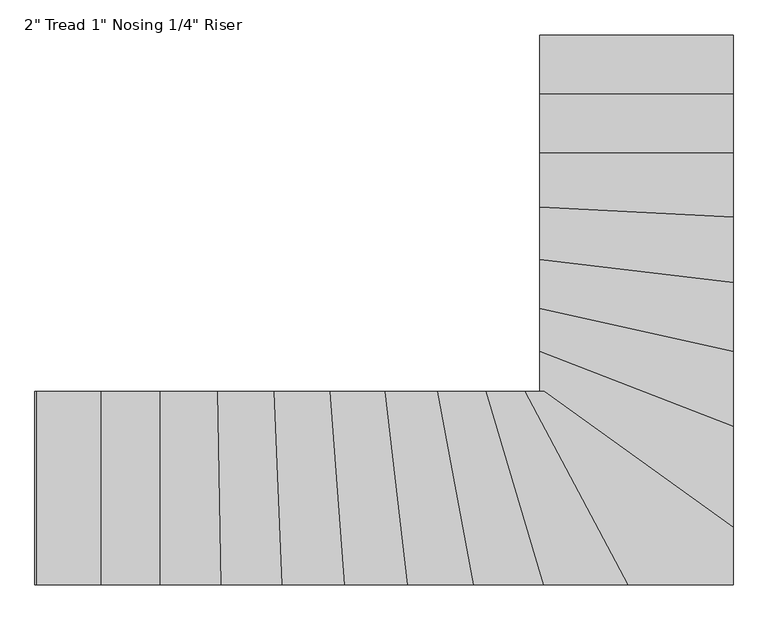
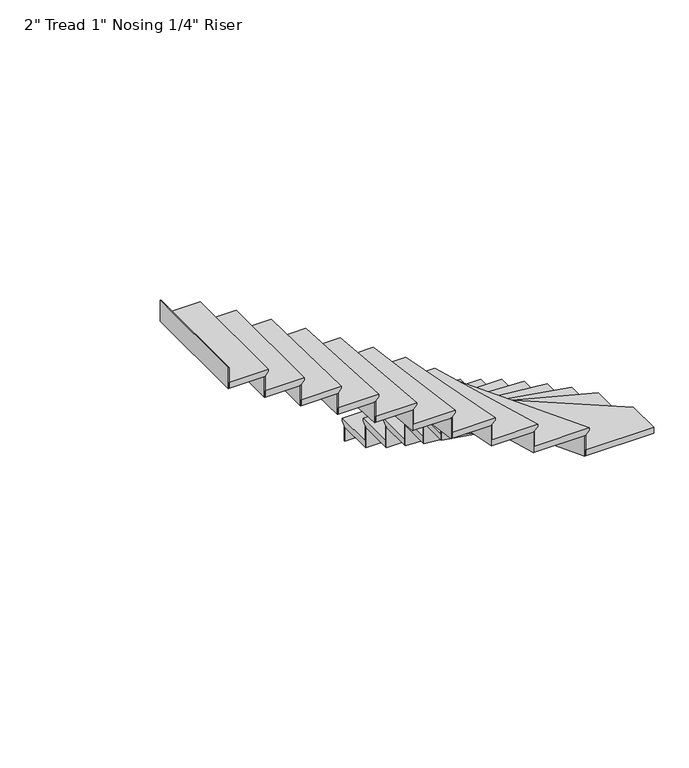
"""IFC4 building model written with IfcOpenShell, lengths in millimetres: stair flight geometry."""

from ifc_helpers import new_model, si_unit, origin, place, context, project, spatial, faceted_brep, source, transform, mapped, element, save


def stair_flight_11d19efb(model_context):
    return source(origin(), model_context, "Body", "Brep", [
        faceted_brep([(541.8084916, 3870.4222402, 3350.6833333), (541.8084916, 3870.4222402, 3369.7333333), (1456.2084916, 3870.4222402, 3369.7333333), (1456.2084916, 3870.4222402, 3350.6833333), (541.8084916, 3845.0222402, 3325.2833333), (1456.2084916, 3845.0222402, 3325.2833333), (541.8084916, 3565.6222402, 3369.7333333), (1456.2084916, 3565.6222402, 3369.7333333), (1456.2084916, 3845.0222402, 3318.9333333), (1456.2084916, 3565.6222402, 3318.9333333), (541.8084916, 3565.6222402, 3318.9333333), (541.8084916, 3845.0222402, 3318.9333333)], [[[0, 1, 2, 3]], [[4, 0, 3, 5]], [[2, 1, 6, 7]], [[8, 9, 10, 11]], [[2, 7, 9, 8, 5, 3]], [[8, 11, 4, 5]], [[6, 1, 0, 4, 11, 10]], [[7, 6, 10, 9]]]),
        faceted_brep([(541.8084916, 3845.0222402, 3318.9333333), (541.8084916, 3845.0222402, 3200.4), (541.8084916, 3838.6722402, 3200.4), (541.8084916, 3838.6722402, 3318.9333333), (1456.2084916, 3845.0222402, 3318.9333333), (1456.2084916, 3838.6722402, 3318.9333333), (1456.2084916, 3838.6722402, 3200.4), (1456.2084916, 3845.0222402, 3200.4)], [[[0, 1, 2, 3]], [[4, 5, 6, 7]], [[1, 0, 4, 7]], [[2, 1, 7, 6]], [[3, 2, 6, 5]], [[0, 3, 5, 4]]]),
        faceted_brep([(541.8084916, 3565.6222402, 3488.2666667), (541.8084916, 3565.6222402, 3318.9333333), (541.8084916, 3559.2722402, 3318.9333333), (541.8084916, 3559.2722402, 3488.2666667), (1456.2084916, 3565.6222402, 3488.2666667), (1456.2084916, 3559.2722402, 3488.2666667), (1456.2084916, 3559.2722402, 3318.9333333), (1456.2084916, 3565.6222402, 3318.9333333)], [[[0, 1, 2, 3]], [[4, 5, 6, 7]], [[1, 0, 4, 7]], [[2, 1, 7, 6]], [[3, 2, 6, 5]], [[0, 3, 5, 4]]]),
        faceted_brep([(1456.2084916, 3591.0222402, 3539.0666667), (541.8084916, 3591.0222402, 3539.0666667), (541.8084916, 3286.2222402, 3539.0666667), (1456.2084916, 3286.2222402, 3539.0666667), (1456.2084916, 3565.6222402, 3488.2666667), (1456.2084916, 3286.2222402, 3488.2666667), (541.8084916, 3286.2222402, 3488.2666667), (541.8084916, 3565.6222402, 3488.2666667), (1456.2084916, 3565.6222402, 3494.6166667), (1456.2084916, 3591.0222402, 3520.0166667), (541.8084916, 3565.6222402, 3494.6166667), (541.8084916, 3591.0222402, 3520.0166667)], [[[0, 1, 2, 3]], [[4, 5, 6, 7]], [[0, 3, 5, 4, 8, 9]], [[4, 7, 10, 8]], [[2, 1, 11, 10, 7, 6]], [[3, 2, 6, 5]], [[11, 1, 0, 9]], [[10, 11, 9, 8]]]),
        faceted_brep([(541.8084916, 3286.2222402, 3657.6), (541.8084916, 3286.2222402, 3488.2666667), (541.8084916, 3279.8722402, 3488.2666667), (541.8084916, 3279.8722402, 3657.6), (1456.2084916, 3286.2222402, 3657.6), (1456.2084916, 3279.8722402, 3657.6), (1456.2084916, 3279.8722402, 3488.2666667), (1456.2084916, 3286.2222402, 3488.2666667)], [[[0, 1, 2, 3]], [[4, 5, 6, 7]], [[1, 0, 4, 7]], [[2, 1, 7, 6]], [[3, 2, 6, 5]], [[0, 3, 5, 4]]]),
        faceted_brep([(1456.2084916, 3311.6222402, 3708.4), (541.8084916, 3311.6222402, 3708.4), (541.8084916, 3029.9557204, 3708.4), (1456.2084916, 2983.6235901, 3708.4), (1456.2084916, 3286.2222402, 3657.6), (1456.2084916, 2983.6235901, 3657.6), (541.8084916, 3029.9557204, 3657.6), (541.8084916, 3286.2222402, 3657.6), (1456.2084916, 3286.2222402, 3663.95), (1456.2084916, 3311.6222402, 3689.35), (541.8084916, 3286.2222402, 3663.95), (541.8084916, 3311.6222402, 3689.35)], [[[0, 1, 2, 3]], [[4, 5, 6, 7]], [[0, 3, 5, 4, 8, 9]], [[4, 7, 10, 8]], [[2, 1, 11, 10, 7, 6]], [[3, 2, 6, 5]], [[11, 1, 0, 9]], [[10, 11, 9, 8]]]),
        faceted_brep([(541.8084916, 3029.9557204, 3826.9333333), (541.8084916, 3029.9557204, 3657.6), (541.8084916, 3023.5975741, 3657.6), (541.8084916, 3023.5975741, 3826.9333333), (1456.2084916, 2983.6235901, 3826.9333333), (1456.2084916, 2977.2654439, 3826.9333333), (1456.2084916, 2977.2654439, 3657.6), (1456.2084916, 2983.6235901, 3657.6)], [[[0, 1, 2, 3]], [[4, 5, 6, 7]], [[1, 0, 4, 7]], [[2, 1, 7, 6]], [[3, 2, 6, 5]], [[0, 3, 5, 4]]]),
        faceted_brep([(1456.2084916, 3009.0561751, 3877.7333333), (541.8084916, 3055.3883053, 3877.7333333), (541.8084916, 2782.3369776, 3877.7333333), (1456.2084916, 2672.1399389, 3877.7333333), (1456.2084916, 2983.6235901, 3826.9333333), (1456.2084916, 2672.1399389, 3826.9333333), (541.8084916, 2782.3369776, 3826.9333333), (541.8084916, 3029.9557204, 3826.9333333), (1456.2084916, 2983.6235901, 3833.2833333), (1456.2084916, 3009.0561751, 3858.6833333), (541.8084916, 3029.9557204, 3833.2833333), (541.8084916, 3055.3883053, 3858.6833333)], [[[0, 1, 2, 3]], [[4, 5, 6, 7]], [[0, 3, 5, 4, 8, 9]], [[4, 7, 10, 8]], [[2, 1, 11, 10, 7, 6]], [[3, 2, 6, 5]], [[11, 1, 0, 9]], [[10, 11, 9, 8]]]),
        faceted_brep([(541.8084916, 2782.3369776, 3996.2666667), (541.8084916, 2782.3369776, 3826.9333333), (541.8084916, 2775.9410322, 3826.9333333), (541.8084916, 2775.9410322, 3996.2666667), (1456.2084916, 2672.1399389, 3996.2666667), (1456.2084916, 2665.7439934, 3996.2666667), (1456.2084916, 2665.7439934, 3826.9333333), (1456.2084916, 2672.1399389, 3826.9333333)], [[[0, 1, 2, 3]], [[4, 5, 6, 7]], [[1, 0, 4, 7]], [[2, 1, 7, 6]], [[3, 2, 6, 5]], [[0, 3, 5, 4]]]),
        faceted_brep([(1456.2084916, 2697.7237208, 4047.0666667), (541.8084916, 2807.9207596, 4047.0666667), (541.8084916, 2549.3331683, 4047.0666667), (1456.2084916, 2345.4640286, 4047.0666667), (1456.2084916, 2672.1399389, 3996.2666667), (1456.2084916, 2345.4640286, 3996.2666667), (541.8084916, 2549.3331683, 3996.2666667), (541.8084916, 2782.3369776, 3996.2666667), (1456.2084916, 2672.1399389, 4002.6166667), (1456.2084916, 2697.7237208, 4028.0166667), (541.8084916, 2782.3369776, 4002.6166667), (541.8084916, 2807.9207596, 4028.0166667)], [[[0, 1, 2, 3]], [[4, 5, 6, 7]], [[0, 3, 5, 4, 8, 9]], [[4, 7, 10, 8]], [[2, 1, 11, 10, 7, 6]], [[3, 2, 6, 5]], [[11, 1, 0, 9]], [[10, 11, 9, 8]]]),
        faceted_brep([(541.8084916, 2549.3331683, 4165.6), (541.8084916, 2549.3331683, 3996.2666667), (541.8084916, 2542.8272579, 3996.2666667), (541.8084916, 2542.8272579, 4165.6), (1456.2084916, 2345.4640286, 4165.6), (1456.2084916, 2338.9581182, 4165.6), (1456.2084916, 2338.9581182, 3996.2666667), (1456.2084916, 2345.4640286, 3996.2666667)], [[[0, 1, 2, 3]], [[4, 5, 6, 7]], [[1, 0, 4, 7]], [[2, 1, 7, 6]], [[3, 2, 6, 5]], [[0, 3, 5, 4]]]),
        faceted_brep([(1456.2084916, 2371.4876703, 4216.4), (541.8084916, 2575.3568101, 4216.4), (541.8084916, 2344.0635087, 4216.4), (1456.2084916, 1989.4955623, 4216.4), (1456.2084916, 2345.4640286, 4165.6), (1456.2084916, 1989.4955623, 4165.6), (541.8084916, 2344.0635087, 4165.6), (541.8084916, 2549.3331683, 4165.6), (1456.2084916, 2345.4640286, 4171.95), (1456.2084916, 2371.4876703, 4197.35), (541.8084916, 2549.3331683, 4171.95), (541.8084916, 2575.3568101, 4197.35)], [[[0, 1, 2, 3]], [[4, 5, 6, 7]], [[0, 3, 5, 4, 8, 9]], [[4, 7, 10, 8]], [[2, 1, 11, 10, 7, 6]], [[3, 2, 6, 5]], [[11, 1, 0, 9]], [[10, 11, 9, 8]]]),
        faceted_brep([(541.8084916, 2344.0635087, 4334.9333333), (541.8084916, 2344.0635087, 4165.6), (541.8084916, 2337.2528325, 4165.6), (541.8084916, 2337.2528325, 4334.9333333), (1456.2084916, 1989.4955623, 4334.9333333), (1456.2084916, 1982.6848861, 4334.9333333), (1456.2084916, 1982.6848861, 4165.6), (1456.2084916, 1989.4955623, 4165.6)], [[[0, 1, 2, 3]], [[4, 5, 6, 7]], [[1, 0, 4, 7]], [[2, 1, 7, 6]], [[3, 2, 6, 5]], [[0, 3, 5, 4]]]),
        faceted_brep([(1456.2084916, 2016.738267, 4385.7333333), (541.8084916, 2371.3062134, 4385.7333333), (541.8084916, 2183.3652728, 4385.7333333), (518.7146085, 2183.3652728, 4385.7333333), (1456.2084916, 1508.8170155, 4385.7333333), (1456.2084916, 1989.4955623, 4334.9333333), (1456.2084916, 1508.8170155, 4334.9333333), (518.7146085, 2183.3652728, 4334.9333333), (541.8084916, 2183.3652728, 4334.9333333), (541.8084916, 2344.0635087, 4334.9333333), (1456.2084916, 1989.4955623, 4341.2833333), (1456.2084916, 2016.738267, 4366.6833333), (541.8084916, 2344.0635087, 4341.2833333), (541.8084916, 2371.3062134, 4366.6833333)], [[[0, 1, 2, 3, 4]], [[5, 6, 7, 8, 9]], [[0, 4, 6, 5, 10, 11]], [[5, 9, 12, 10]], [[2, 1, 13, 12, 9, 8]], [[4, 3, 7, 6]], [[13, 1, 0, 11]], [[12, 13, 11, 10]], [[3, 2, 8, 7]]]),
        faceted_brep([(518.7146085, 2183.3652728, 4504.2666667), (518.7146085, 2183.3652728, 4334.9333333), (507.8422444, 2183.3652728, 4334.9333333), (507.8422444, 2183.3652728, 4504.2666667), (1456.2084916, 1508.8170155, 4504.2666667), (1456.2084916, 1500.9941013, 4504.2666667), (1456.2084916, 1500.9941013, 4334.9333333), (1456.2084916, 1508.8170155, 4334.9333333)], [[[0, 1, 2, 3]], [[4, 5, 6, 7]], [[1, 0, 4, 7]], [[2, 1, 7, 6]], [[3, 2, 6, 5]], [[0, 3, 5, 4]]]),
        faceted_brep([(928.7056408, 1268.9652728, 4555.0666667), (1456.2084916, 1268.9652728, 4555.0666667), (1456.2084916, 1540.1086724, 4555.0666667), (562.2040648, 2183.3652728, 4555.0666667), (442.5531734, 2183.3652728, 4555.0666667), (1456.2084916, 1268.9652728, 4504.2666667), (928.7056408, 1268.9652728, 4504.2666667), (442.5531734, 2183.3652728, 4504.2666667), (518.7146085, 2183.3652728, 4504.2666667), (1456.2084916, 1508.8170155, 4504.2666667), (518.7146085, 2183.3652728, 4510.6166667), (1456.2084916, 1508.8170155, 4510.6166667), (562.2040648, 2183.3652728, 4536.0166667), (1456.2084916, 1540.1086724, 4536.0166667)], [[[0, 1, 2, 3, 4]], [[5, 6, 7, 8, 9]], [[1, 0, 6, 5]], [[9, 8, 10, 11]], [[0, 4, 7, 6]], [[12, 3, 2, 13]], [[10, 12, 13, 11]], [[2, 1, 5, 9, 11, 13]], [[4, 3, 12, 10, 8, 7]]]),
        faceted_brep([(442.5531734, 2183.3652728, 4673.6), (442.5531734, 2183.3652728, 4504.2666667), (435.3614926, 2183.3652728, 4504.2666667), (435.3614926, 2183.3652728, 4673.6), (928.7056408, 1268.9652728, 4673.6), (921.51396, 1268.9652728, 4673.6), (921.51396, 1268.9652728, 4504.2666667), (928.7056408, 1268.9652728, 4504.2666667)], [[[0, 1, 2, 3]], [[4, 5, 6, 7]], [[1, 0, 4, 7]], [[2, 1, 7, 6]], [[3, 2, 6, 5]], [[0, 3, 5, 4]]]),
        faceted_brep([(957.4723641, 1268.9652728, 4724.4), (471.3198967, 2183.3652728, 4724.4), (259.1852093, 2183.3652728, 4724.4), (530.810737, 1268.9652728, 4724.4), (928.7056408, 1268.9652728, 4673.6), (530.810737, 1268.9652728, 4673.6), (259.1852093, 2183.3652728, 4673.6), (442.5531734, 2183.3652728, 4673.6), (928.7056408, 1268.9652728, 4679.95), (957.4723641, 1268.9652728, 4705.35), (442.5531734, 2183.3652728, 4679.95), (471.3198967, 2183.3652728, 4705.35)], [[[0, 1, 2, 3]], [[4, 5, 6, 7]], [[0, 3, 5, 4, 8, 9]], [[4, 7, 10, 8]], [[2, 1, 11, 10, 7, 6]], [[3, 2, 6, 5]], [[11, 1, 0, 9]], [[10, 11, 9, 8]]]),
        faceted_brep([(259.1852093, 2183.3652728, 4842.9333333), (259.1852093, 2183.3652728, 4673.6), (252.5609672, 2183.3652728, 4673.6), (252.5609672, 2183.3652728, 4842.9333333), (530.810737, 1268.9652728, 4842.9333333), (524.1864949, 1268.9652728, 4842.9333333), (524.1864949, 1268.9652728, 4673.6), (530.810737, 1268.9652728, 4673.6)], [[[0, 1, 2, 3]], [[4, 5, 6, 7]], [[1, 0, 4, 7]], [[2, 1, 7, 6]], [[3, 2, 6, 5]], [[0, 3, 5, 4]]]),
        faceted_brep([(557.3077055, 1268.9652728, 4893.7333333), (285.6821779, 2183.3652728, 4893.7333333), (32.036519, 2183.3652728, 4893.7333333), (200.498444, 1268.9652728, 4893.7333333), (530.810737, 1268.9652728, 4842.9333333), (200.498444, 1268.9652728, 4842.9333333), (32.036519, 2183.3652728, 4842.9333333), (259.1852093, 2183.3652728, 4842.9333333), (530.810737, 1268.9652728, 4849.2833333), (557.3077055, 1268.9652728, 4874.6833333), (259.1852093, 2183.3652728, 4849.2833333), (285.6821779, 2183.3652728, 4874.6833333)], [[[0, 1, 2, 3]], [[4, 5, 6, 7]], [[0, 3, 5, 4, 8, 9]], [[4, 7, 10, 8]], [[2, 1, 11, 10, 7, 6]], [[3, 2, 6, 5]], [[11, 1, 0, 9]], [[10, 11, 9, 8]]]),
        faceted_brep([(32.036519, 2183.3652728, 5012.2666667), (32.036519, 2183.3652728, 4842.9333333), (25.579654, 2183.3652728, 4842.9333333), (25.579654, 2183.3652728, 5012.2666667), (200.498444, 1268.9652728, 5012.2666667), (194.0415789, 1268.9652728, 5012.2666667), (194.0415789, 1268.9652728, 4842.9333333), (200.498444, 1268.9652728, 4842.9333333)], [[[0, 1, 2, 3]], [[4, 5, 6, 7]], [[1, 0, 4, 7]], [[2, 1, 7, 6]], [[3, 2, 6, 5]], [[0, 3, 5, 4]]]),
        faceted_brep([(226.3259042, 1268.9652728, 5063.0666667), (57.8639792, 2183.3652728, 5063.0666667), (-216.5399099, 2183.3652728, 5063.0666667), (-109.2188993, 1268.9652728, 5063.0666667), (200.498444, 1268.9652728, 5012.2666667), (-109.2188993, 1268.9652728, 5012.2666667), (-216.5399099, 2183.3652728, 5012.2666667), (32.036519, 2183.3652728, 5012.2666667), (200.498444, 1268.9652728, 5018.6166667), (226.3259042, 1268.9652728, 5044.0166667), (32.036519, 2183.3652728, 5018.6166667), (57.8639792, 2183.3652728, 5044.0166667)], [[[0, 1, 2, 3]], [[4, 5, 6, 7]], [[0, 3, 5, 4, 8, 9]], [[4, 7, 10, 8]], [[2, 1, 11, 10, 7, 6]], [[3, 2, 6, 5]], [[11, 1, 0, 9]], [[10, 11, 9, 8]]]),
        faceted_brep([(-216.5399099, 2183.3652728, 5181.6), (-216.5399099, 2183.3652728, 5012.2666667), (-222.9334965, 2183.3652728, 5012.2666667), (-222.9334965, 2183.3652728, 5181.6), (-109.2188993, 1268.9652728, 5181.6), (-115.6124859, 1268.9652728, 5181.6), (-115.6124859, 1268.9652728, 5012.2666667), (-109.2188993, 1268.9652728, 5012.2666667)], [[[0, 1, 2, 3]], [[4, 5, 6, 7]], [[1, 0, 4, 7]], [[2, 1, 7, 6]], [[3, 2, 6, 5]], [[0, 3, 5, 4]]]),
        faceted_brep([(-83.644553, 1268.9652728, 5232.4), (-190.9655636, 2183.3652728, 5232.4), (-475.6084446, 2183.3652728, 5232.4), (-408.7373342, 1268.9652728, 5232.4), (-109.2188993, 1268.9652728, 5181.6), (-408.7373342, 1268.9652728, 5181.6), (-475.6084446, 2183.3652728, 5181.6), (-216.5399099, 2183.3652728, 5181.6), (-109.2188993, 1268.9652728, 5187.95), (-83.644553, 1268.9652728, 5213.35), (-216.5399099, 2183.3652728, 5187.95), (-190.9655636, 2183.3652728, 5213.35)], [[[0, 1, 2, 3]], [[4, 5, 6, 7]], [[0, 3, 5, 4, 8, 9]], [[4, 7, 10, 8]], [[2, 1, 11, 10, 7, 6]], [[3, 2, 6, 5]], [[11, 1, 0, 9]], [[10, 11, 9, 8]]]),
        faceted_brep([(-475.6084446, 2183.3652728, 5350.9333333), (-475.6084446, 2183.3652728, 5181.6), (-481.9754023, 2183.3652728, 5181.6), (-481.9754023, 2183.3652728, 5350.9333333), (-408.7373342, 1268.9652728, 5350.9333333), (-415.104292, 1268.9652728, 5350.9333333), (-415.104292, 1268.9652728, 5181.6), (-408.7373342, 1268.9652728, 5181.6)], [[[0, 1, 2, 3]], [[4, 5, 6, 7]], [[1, 0, 4, 7]], [[2, 1, 7, 6]], [[3, 2, 6, 5]], [[0, 3, 5, 4]]]),
        faceted_brep([(-383.2695031, 1268.9652728, 5401.7333333), (-450.1406135, 2183.3652728, 5401.7333333), (-740.5916411, 2183.3652728, 5401.7333333), (-702.4626207, 1268.9652728, 5401.7333333), (-408.7373342, 1268.9652728, 5350.9333333), (-702.4626207, 1268.9652728, 5350.9333333), (-740.5916411, 2183.3652728, 5350.9333333), (-475.6084446, 2183.3652728, 5350.9333333), (-408.7373342, 1268.9652728, 5357.2833333), (-383.2695031, 1268.9652728, 5382.6833333), (-475.6084446, 2183.3652728, 5357.2833333), (-450.1406135, 2183.3652728, 5382.6833333)], [[[0, 1, 2, 3]], [[4, 5, 6, 7]], [[0, 3, 5, 4, 8, 9]], [[4, 7, 10, 8]], [[2, 1, 11, 10, 7, 6]], [[3, 2, 6, 5]], [[11, 1, 0, 9]], [[10, 11, 9, 8]]]),
        faceted_brep([(-740.5916411, 2183.3652728, 5520.2666667), (-740.5916411, 2183.3652728, 5350.9333333), (-746.9471593, 2183.3652728, 5350.9333333), (-746.9471593, 2183.3652728, 5520.2666667), (-702.4626207, 1268.9652728, 5520.2666667), (-708.8181389, 1268.9652728, 5520.2666667), (-708.8181389, 1268.9652728, 5350.9333333), (-702.4626207, 1268.9652728, 5350.9333333)], [[[0, 1, 2, 3]], [[4, 5, 6, 7]], [[1, 0, 4, 7]], [[2, 1, 7, 6]], [[3, 2, 6, 5]], [[0, 3, 5, 4]]]),
        faceted_brep([(-677.0405481, 1268.9652728, 5571.0666667), (-715.1695685, 2183.3652728, 5571.0666667), (-1009.2364216, 2183.3652728, 5571.0666667), (-992.5821201, 1268.9652728, 5571.0666667), (-702.4626207, 1268.9652728, 5520.2666667), (-992.5821201, 1268.9652728, 5520.2666667), (-1009.2364216, 2183.3652728, 5520.2666667), (-740.5916411, 2183.3652728, 5520.2666667), (-702.4626207, 1268.9652728, 5526.6166667), (-677.0405481, 1268.9652728, 5552.0166667), (-740.5916411, 2183.3652728, 5526.6166667), (-715.1695685, 2183.3652728, 5552.0166667)], [[[0, 1, 2, 3]], [[4, 5, 6, 7]], [[0, 3, 5, 4, 8, 9]], [[4, 7, 10, 8]], [[2, 1, 11, 10, 7, 6]], [[3, 2, 6, 5]], [[11, 1, 0, 9]], [[10, 11, 9, 8]]]),
        faceted_brep([(-1009.2364216, 2183.3652728, 5689.6), (-1009.2364216, 2183.3652728, 5520.2666667), (-1015.5874748, 2183.3652728, 5520.2666667), (-1015.5874748, 2183.3652728, 5689.6), (-992.5821201, 1268.9652728, 5689.6), (-998.9331733, 1268.9652728, 5689.6), (-998.9331733, 1268.9652728, 5520.2666667), (-992.5821201, 1268.9652728, 5520.2666667)], [[[0, 1, 2, 3]], [[4, 5, 6, 7]], [[1, 0, 4, 7]], [[2, 1, 7, 6]], [[3, 2, 6, 5]], [[0, 3, 5, 4]]]),
        faceted_brep([(-967.1779075, 1268.9652728, 5740.4), (-983.832209, 2183.3652728, 5740.4), (-1280.3050583, 2183.3652728, 5740.4), (-1280.3050583, 1268.9652728, 5740.4), (-992.5821201, 1268.9652728, 5689.6), (-1280.3050583, 1268.9652728, 5689.6), (-1280.3050583, 2183.3652728, 5689.6), (-1009.2364216, 2183.3652728, 5689.6), (-992.5821201, 1268.9652728, 5695.95), (-967.1779075, 1268.9652728, 5721.35), (-1009.2364216, 2183.3652728, 5695.95), (-983.832209, 2183.3652728, 5721.35)], [[[0, 1, 2, 3]], [[4, 5, 6, 7]], [[0, 3, 5, 4, 8, 9]], [[4, 7, 10, 8]], [[2, 1, 11, 10, 7, 6]], [[3, 2, 6, 5]], [[11, 1, 0, 9]], [[10, 11, 9, 8]]]),
        faceted_brep([(-1280.3050583, 2183.3652728, 5858.9333333), (-1280.3050583, 2183.3652728, 5689.6), (-1286.6550583, 2183.3652728, 5689.6), (-1286.6550583, 2183.3652728, 5858.9333333), (-1280.3050583, 1268.9652728, 5858.9333333), (-1286.6550583, 1268.9652728, 5858.9333333), (-1286.6550583, 1268.9652728, 5689.6), (-1280.3050583, 1268.9652728, 5689.6)], [[[0, 1, 2, 3]], [[4, 5, 6, 7]], [[1, 0, 4, 7]], [[2, 1, 7, 6]], [[3, 2, 6, 5]], [[0, 3, 5, 4]]]),
        faceted_brep([(-1254.9050583, 1268.9652728, 5909.7333333), (-1254.9050583, 2183.3652728, 5909.7333333), (-1559.7050583, 2183.3652728, 5909.7333333), (-1559.7050583, 1268.9652728, 5909.7333333), (-1280.3050583, 1268.9652728, 5858.9333333), (-1559.7050583, 1268.9652728, 5858.9333333), (-1559.7050583, 2183.3652728, 5858.9333333), (-1280.3050583, 2183.3652728, 5858.9333333), (-1280.3050583, 1268.9652728, 5865.2833333), (-1254.9050583, 1268.9652728, 5890.6833333), (-1280.3050583, 2183.3652728, 5865.2833333), (-1254.9050583, 2183.3652728, 5890.6833333)], [[[0, 1, 2, 3]], [[4, 5, 6, 7]], [[0, 3, 5, 4, 8, 9]], [[4, 7, 10, 8]], [[2, 1, 11, 10, 7, 6]], [[3, 2, 6, 5]], [[11, 1, 0, 9]], [[10, 11, 9, 8]]]),
        faceted_brep([(-1559.7050583, 2183.3652728, 6028.2666667), (-1559.7050583, 2183.3652728, 5858.9333333), (-1566.0550583, 2183.3652728, 5858.9333333), (-1566.0550583, 2183.3652728, 6028.2666667), (-1559.7050583, 1268.9652728, 6028.2666667), (-1566.0550583, 1268.9652728, 6028.2666667), (-1566.0550583, 1268.9652728, 5858.9333333), (-1559.7050583, 1268.9652728, 5858.9333333)], [[[0, 1, 2, 3]], [[4, 5, 6, 7]], [[1, 0, 4, 7]], [[2, 1, 7, 6]], [[3, 2, 6, 5]], [[0, 3, 5, 4]]]),
        faceted_brep([(-1839.1050583, 2183.3652728, 6197.6), (-1839.1050583, 2183.3652728, 6028.2666667), (-1845.4550583, 2183.3652728, 6028.2666667), (-1845.4550583, 2183.3652728, 6197.6), (-1839.1050583, 1268.9652728, 6197.6), (-1845.4550583, 1268.9652728, 6197.6), (-1845.4550583, 1268.9652728, 6028.2666667), (-1839.1050583, 1268.9652728, 6028.2666667)], [[[0, 1, 2, 3]], [[4, 5, 6, 7]], [[1, 0, 4, 7]], [[2, 1, 7, 6]], [[3, 2, 6, 5]], [[0, 3, 5, 4]]]),
        faceted_brep([(-1534.3050583, 1268.9652728, 6079.0666667), (-1534.3050583, 2183.3652728, 6079.0666667), (-1839.1050583, 2183.3652728, 6079.0666667), (-1839.1050583, 1268.9652728, 6079.0666667), (-1559.7050583, 1268.9652728, 6028.2666667), (-1839.1050583, 1268.9652728, 6028.2666667), (-1839.1050583, 2183.3652728, 6028.2666667), (-1559.7050583, 2183.3652728, 6028.2666667), (-1559.7050583, 1268.9652728, 6034.6166667), (-1534.3050583, 1268.9652728, 6060.0166667), (-1559.7050583, 2183.3652728, 6034.6166667), (-1534.3050583, 2183.3652728, 6060.0166667)], [[[0, 1, 2, 3]], [[4, 5, 6, 7]], [[0, 3, 5, 4, 8, 9]], [[4, 7, 10, 8]], [[2, 1, 11, 10, 7, 6]], [[3, 2, 6, 5]], [[11, 1, 0, 9]], [[10, 11, 9, 8]]]),
    ])


if __name__ == "__main__":
    model = new_model("IFC4")
    model_context = context("Model", 3, world=origin())
    ifc_project = project(units=[si_unit("LENGTHUNIT", "METRE", prefix="MILLI")], contexts=[model_context])
    site = spatial("IfcSite", under=ifc_project)
    building = spatial("IfcBuilding", under=site)
    placement = place(None, origin())
    stair_flight_shape = stair_flight_11d19efb(model_context)
    element("IfcStairFlight", 1, ObjectType="2\" Tread 1\" Nosing 1/4\" Riser", at=placement, inside=building, context=model_context, shape_type="MappedRepresentation", body=[
        mapped(stair_flight_shape, transform((0.0, 0.0, 0.0), x_axis=(1.0, 0.0, 0.0), y_axis=(0.0, 1.0, 0.0), z_axis=(0.0, 0.0, 1.0))),
    ])
    save(model, "model.ifc")
